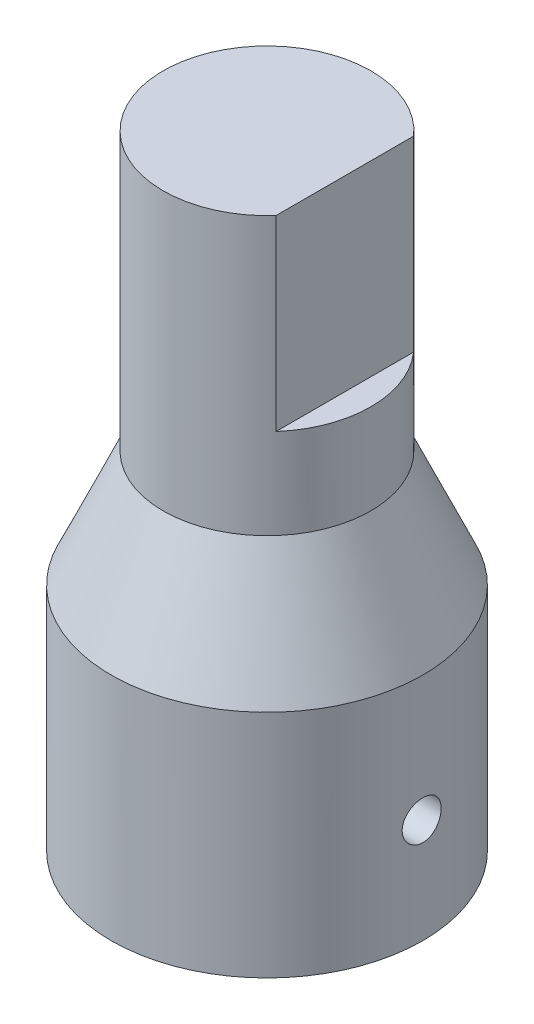
from build123d import *

# Parameters (mm, degrees)
BASE_CYLINDER_SKETCH_19_05_R = 9.525
BASE_CYLINDER_19_05_DEPTH    = 14.06
TAPER_TOP_SKETCH_12_7_R      = 6.35
SHANK_SKETCH_R               = 6.35
SHANK_12_7_DEPTH             = 16.94
SHANK_FLAT_SKETCH_W          = 1.59
SHANK_FLAT_SKETCH_H          = 11.43
SHANK_FLAT_DEPTH             = 8.47
BORE_SKETCH_11_11_R          = 6.35
BORE_11_11_DEPTH             = 14.06
CROSS_HOLE_SKETCH_2_38_R     = 1.19
CROSS_HOLE_2_38_DEPTH        = 14.06


with BuildPart() as part:
    # Base Cylinder Sketch Ø19.05 → Base Cylinder Ø19.05 (new body)
    with BuildSketch(Plane(origin=(0, 0, 0), x_dir=(1, 0, 0), z_dir=(0, 1, 0))):
        with Locations(Location((0, 0, 0), (0, 0, 270))):
            Circle(BASE_CYLINDER_SKETCH_19_05_R)
    extrude(amount=BASE_CYLINDER_19_05_DEPTH)

    # Taper Top Sketch Ø12.7 → section 0 of taper_loft
    with BuildSketch(Plane(origin=(0, 21.16, 0), x_dir=(1, 0, 0), z_dir=(0, 1, 0)), mode=Mode.PRIVATE) as taper_loft_s0:
        Circle(TAPER_TOP_SKETCH_12_7_R)
    # loft up to a face of the part (taper_loft)
    loft([taper_loft_s0.sketch, Face(Wire([part.edges().sort_by_distance((6.943426176, 14.06, -6.520311184))[0]]))])

    # Shank Sketch → Shank Ø12.7 (add)
    with BuildSketch(Plane(origin=(0, 21.16, 0), x_dir=(1, 0, 0), z_dir=(0, 1, 0))):
        with Locations(Location((0, 0, 0), (0, 0, 270))):
            Circle(SHANK_SKETCH_R)
    extrude(amount=SHANK_12_7_DEPTH)

    # Shank Flat Sketch → Shank Flat (cut, symmetric)
    with BuildSketch(Plane.XY):
        with Locations((5.555, 32.385)):
            Rectangle(SHANK_FLAT_SKETCH_W, SHANK_FLAT_SKETCH_H)
    extrude(amount=SHANK_FLAT_DEPTH, both=True, mode=Mode.SUBTRACT)

    # Bore Sketch Ø11.11 → Bore Ø11.11 (cut)
    with BuildSketch(Plane.XZ):
        with Locations(Location((0, 0, 0), (0, 0, 270))):
            Circle(BORE_SKETCH_11_11_R)
    extrude(amount=-BORE_11_11_DEPTH, mode=Mode.SUBTRACT)

    # Cross Hole Sketch Ø2.38 → Cross Hole Ø2.38 (cut)
    with BuildSketch(Plane(origin=(0, 0, 0), x_dir=(0, 0, -1), z_dir=(1, 0, 0))):
        with Locations(Location((0, 6.38, 0), (0, 0, 180))):
            Circle(CROSS_HOLE_SKETCH_2_38_R)
    extrude(amount=CROSS_HOLE_2_38_DEPTH, mode=Mode.SUBTRACT)


solid = part.part
